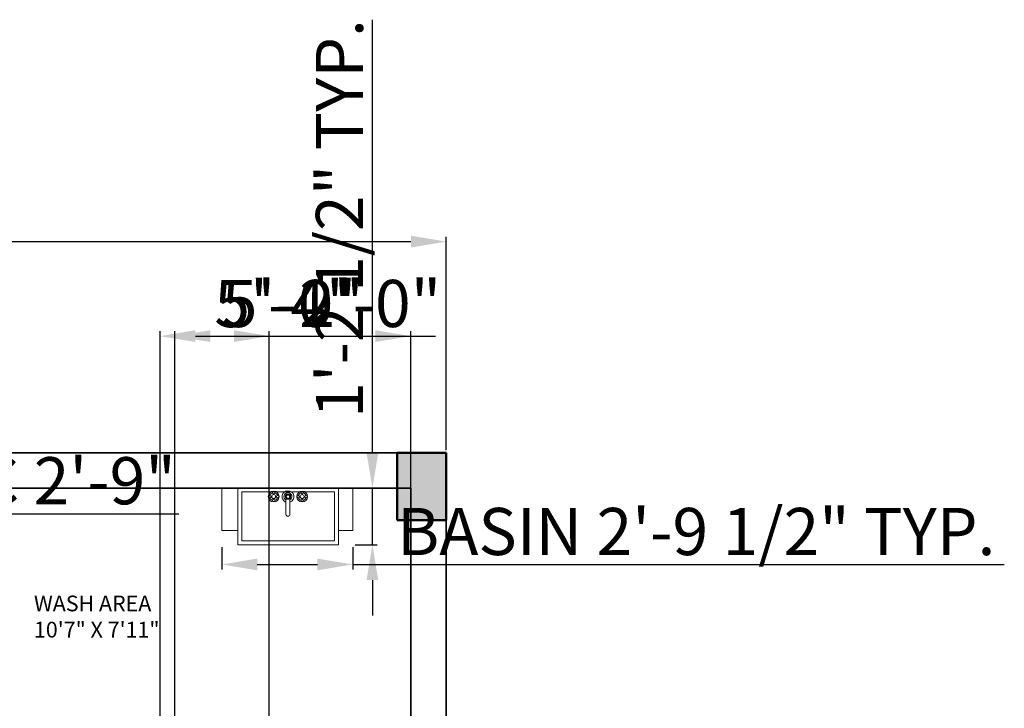
# Model space of a CAD drawing. Units: inches. Extents: x 1132 to 1713, y 3115 to 3781.
# Tile 4 of 4: x 1455 to 1705, y 3606 to 3781. Entities that reach past the tile are written whole.
import ezdxf

# ---------------------------------------------------------------- set-up
doc = ezdxf.new("R2010")
doc.units = ezdxf.units.IN
for name, color, linetype, lineweight in [('A-ANNO-DIMS', 2, 'Continuous', 18), ('A-AREA-IDEN', 7, 'Continuous', 18), ('A-COLS', 1, 'Continuous', 50), ('A-COLS-PATT', 252, 'Continuous', 13), ('A-FLOR-FIXT', 9, 'Continuous', 18), ('A-WALL', 7, 'Continuous', 35)]:
    doc.layers.add(name, color=color, linetype=linetype, lineweight=lineweight)
doc.styles.get("Standard").update_dxf_attribs({"font": 'arial.ttf'})
doc.dimstyles.new('ISO-25', dxfattribs={"dimtxt": 12, "dimasz": 9, "dimexe": 1.25, "dimexo": 0.625, "dimtad": 1, "dimdec": 0, "dimrnd": 2, "dimlunit": 3, "dimtxsty": 'Standard', "dimcen": 2.5, "dimadec": 0, "dimazin": 0, "dimtfac": 1, "dimtdec": 0, "dimtmove": 0, "dimatfit": 3, "dimfxl": 1, "dimarcsym": 0})

# ---------------------------------------------------------------- blocks, each defined once
blk = doc.blocks.new('*D19')
at = {"layer": 'A-ANNO-DIMS', "color": 0, "lineweight": -2, "transparency": 16777216}
for p, q in [((1268.16, 3667), (1268.16, 3725.86)), ((1563.22, 3671.51), (1563.22, 3725.86)), ((1277.16, 3724.61), (1554.22, 3724.61))]:
    blk.add_line(p, q, dxfattribs=at)
at = {"layer": 'A-ANNO-DIMS', "color": 0, "transparency": 16777216}
for points in [[(1277.16, 3726.11), (1277.16, 3723.11), (1268.16, 3724.61)], [(1554.22, 3726.11), (1554.22, 3723.11), (1563.22, 3724.61)]]:
    blk.add_solid(points, dxfattribs=at)
at = {"layer": 'Defpoints', "color": 0, "transparency": 16777216}
for p in [(1563.22, 3724.61), (1563.22, 3670.89), (1268.16, 3666.38)]:
    blk.add_point(p, dxfattribs=at)
at = {"layer": 'A-ANNO-DIMS', "color": 0, "transparency": 16777216, "insert": (1415.69, 3731.36), "char_height": 12, "attachment_point": 5}
blk.add_mtext('24\'-8"', dxfattribs=at)
blk = doc.blocks.new('Faucet - Bathroom top')
for p, q in [((-4.107, 0.125), (-4.375, 0.125)), ((-3.75, 0.4788), (-3.75, 0.75)), ((-3.5, 0.482), (-3.5, 0.75)), ((-3.1461, 0.125), (-2.875, 0.125)), ((3.143, 0.125), (2.875, 0.125)), ((3.5, 0.4788), (3.5, 0.75)), ((3.75, 0.482), (3.75, 0.75)), ((4.1039, 0.125), (4.375, 0.125)), ((-4.1039, -0.125), (-4.375, -0.125)), ((-3.75, -0.4821), (-3.75, -0.75)), ((-3.5, -0.4789), (-3.5, -0.75)), ((-3.143, -0.125), (-2.875, -0.125)), ((-0.5, -0.8639), (-0.5, -4.5)), ((0.5, -4.5), (0.5, -0.8631)), ((3.1461, -0.125), (2.875, -0.125)), ((3.5, -0.4821), (3.5, -0.75)), ((3.75, -0.4789), (3.75, -0.75)), ((4.107, -0.125), (4.375, -0.125))]:
    blk.add_line(p, q)
for centre, radius in [((-3.625, 0), 1.375), ((-4.625, 0), 0.2795), ((-3.625, 0), 0.5), ((-3.625, 1), 0.2795), ((-2.625, 0), 0.2795), ((0, 0), 0.5), ((3.625, 0), 1.375), ((2.625, 0), 0.2795), ((3.625, 0), 0.5), ((3.625, 1), 0.2795), ((4.625, 0), 0.2795), ((-3.625, -1), 0.2795), ((3.625, -1), 0.2795)]:
    blk.add_circle(centre, radius)
for centre, radius, start, end in [((-3.625, 0), 1, 105.2407, 164.2093), ((-3.625, 0), 1, 16.44125, 74.07887), ((0, 0), 1.5, 289.6514, 250.3603), ((0, 0), 1, 300.3431, 239.7554), ((3.625, 0), 1, 106.12, 164.0884), ((3.625, 0), 1, 16.23422, 73.90469), ((-3.625, 0), 1, 196.2342, 253.9047), ((-3.625, 0), 1, 286.12, 344.0884), ((3.625, 0), 1, 196.4413, 254.0789), ((3.625, 0), 1, 285.2407, 344.2093), ((0, -4.5), 0.5, 180, 0)]:
    blk.add_arc(centre, radius, start, end)
blk = doc.blocks.new('LAVATORY-WALL-MOUNT')
for p, q in [((-16.8, 2.17), (-16.8, -8.61)), ((16.5, -8.61), (16.5, 2.17)), ((-16.8, -8.61), (-12.71, -8.61)), ((12.88, -8.61), (16.5, -8.61))]:
    blk.add_line(p, q)
for points in [[(-12.71, 2.17), (12.88, 2.17), (12.88, -12.27), (-12.71, -12.27)], [(-11.71, 1.17), (11.88, 1.17), (11.88, -11.27), (-11.71, -11.27)]]:
    blk.add_lwpolyline(points, close=True)
for radius in [0.667, 0.447]:
    blk.add_circle((0, 0), radius)
blk.add_blockref('Faucet - Bathroom top', (0, 0))
blk = doc.blocks.new('*D28')
at = {"layer": 'A-ANNO-DIMS', "color": 0, "lineweight": -2, "transparency": 16777216}
for p, q in [((1506.13, 3646.81), (1506.13, 3641.19)), ((1539.42, 3646.81), (1539.42, 3641.19)), ((1515.13, 3642.44), (1530.42, 3642.44)), ((1539.42, 3642.44), (1705.22, 3642.44))]:
    blk.add_line(p, q, dxfattribs=at)
at = {"layer": 'A-ANNO-DIMS', "color": 0, "transparency": 16777216}
for points in [[(1515.13, 3643.94), (1515.13, 3640.94), (1506.13, 3642.44)], [(1530.42, 3643.94), (1530.42, 3640.94), (1539.42, 3642.44)]]:
    blk.add_solid(points, dxfattribs=at)
at = {"layer": 'Defpoints', "color": 0, "transparency": 16777216}
for p in [(1506.13, 3647.44), (1539.42, 3647.44), (1539.42, 3642.44)]:
    blk.add_point(p, dxfattribs=at)
at = {"layer": 'A-ANNO-DIMS', "color": 0, "transparency": 16777216, "insert": (1626.82, 3649.27), "char_height": 12, "attachment_point": 5}
blk.add_mtext('BASIN 2\'-9 1/2" TYP.', dxfattribs=at)
blk = doc.blocks.new('*D29')
at = {"layer": 'A-ANNO-DIMS', "color": 0, "lineweight": -2, "transparency": 16777216}
for p, q in [((1544.42, 3670.88), (1544.42, 3781.1)), ((1540.05, 3661.88), (1545.67, 3661.88)), ((1544.42, 3647.44), (1544.42, 3661.88)), ((1540.05, 3647.44), (1545.67, 3647.44)), ((1544.42, 3638.44), (1544.42, 3629.44))]:
    blk.add_line(p, q, dxfattribs=at)
at = {"layer": 'A-ANNO-DIMS', "color": 0, "transparency": 16777216}
for points in [[(1542.92, 3670.88), (1545.92, 3670.88), (1544.42, 3661.88)], [(1542.92, 3638.44), (1545.92, 3638.44), (1544.42, 3647.44)]]:
    blk.add_solid(points, dxfattribs=at)
at = {"layer": 'Defpoints', "color": 0, "transparency": 16777216}
for p in [(1539.42, 3661.88), (1544.42, 3661.88), (1539.42, 3647.44)]:
    blk.add_point(p, dxfattribs=at)
at = {"layer": 'A-ANNO-DIMS', "color": 0, "transparency": 16777216, "insert": (1537.59, 3730.49), "char_height": 12, "attachment_point": 5, "rotation": 90}
blk.add_mtext('1\'-2 1/2" TYP.', dxfattribs=at)
blk = doc.blocks.new('*D36')
at = {"layer": 'A-ANNO-DIMS', "color": 0, "lineweight": -2, "transparency": 16777216}
for p, q in [((1386.9, 3651.03), (1386.9, 3656.61)), ((1419.95, 3651.03), (1419.95, 3656.61)), ((1395.9, 3655.36), (1410.95, 3655.36)), ((1419.95, 3655.36), (1495.17, 3655.36))]:
    blk.add_line(p, q, dxfattribs=at)
at = {"layer": 'A-ANNO-DIMS', "color": 0, "transparency": 16777216}
for points in [[(1395.9, 3656.86), (1395.9, 3653.86), (1386.9, 3655.36)], [(1410.95, 3656.86), (1410.95, 3653.86), (1419.95, 3655.36)]]:
    blk.add_solid(points, dxfattribs=at)
at = {"layer": 'Defpoints', "color": 0, "transparency": 16777216}
for p in [(1419.95, 3655.36), (1386.9, 3650.4), (1419.95, 3650.4)]:
    blk.add_point(p, dxfattribs=at)
at = {"layer": 'A-ANNO-DIMS', "color": 0, "transparency": 16777216, "insert": (1462.06, 3662.19), "char_height": 12, "attachment_point": 5}
blk.add_mtext('WC 2\'-9"', dxfattribs=at)
blk = doc.blocks.new('*D50')
at = {"layer": 'A-ANNO-DIMS', "color": 0, "lineweight": -2, "transparency": 16777216}
for p, q in [((1490.38, 3260.74), (1490.38, 3701.81)), ((1554.16, 3217.5), (1554.16, 3701.81)), ((1499.38, 3700.56), (1545.16, 3700.56))]:
    blk.add_line(p, q, dxfattribs=at)
at = {"layer": 'A-ANNO-DIMS', "color": 0, "transparency": 16777216}
for points in [[(1499.38, 3702.06), (1499.38, 3699.06), (1490.38, 3700.56)], [(1545.16, 3702.06), (1545.16, 3699.06), (1554.16, 3700.56)]]:
    blk.add_solid(points, dxfattribs=at)
at = {"layer": 'Defpoints', "color": 0, "transparency": 16777216}
for p in [(1554.16, 3700.56), (1490.38, 3260.12), (1554.16, 3216.88)]:
    blk.add_point(p, dxfattribs=at)
at = {"layer": 'A-ANNO-DIMS', "color": 0, "transparency": 16777216, "insert": (1522.27, 3707.29), "char_height": 12, "attachment_point": 5}
blk.add_mtext('5\'-4"', dxfattribs=at)
blk = doc.blocks.new('*D55')
at = {"layer": 'A-ANNO-DIMS', "color": 0, "lineweight": -2, "transparency": 16777216}
for p, q in [((1494.16, 3463.5), (1494.16, 3701.81)), ((1554.16, 3463.5), (1554.16, 3701.81)), ((1503.16, 3700.56), (1545.16, 3700.56))]:
    blk.add_line(p, q, dxfattribs=at)
at = {"layer": 'A-ANNO-DIMS', "color": 0, "transparency": 16777216}
for points in [[(1503.16, 3702.06), (1503.16, 3699.06), (1494.16, 3700.56)], [(1545.16, 3702.06), (1545.16, 3699.06), (1554.16, 3700.56)]]:
    blk.add_solid(points, dxfattribs=at)
at = {"layer": 'Defpoints', "color": 0, "transparency": 16777216}
for p in [(1554.16, 3700.56), (1494.16, 3462.88), (1554.16, 3462.88)]:
    blk.add_point(p, dxfattribs=at)
at = {"layer": 'A-ANNO-DIMS', "color": 0, "transparency": 16777216, "insert": (1524.16, 3707.31), "char_height": 12, "attachment_point": 5}
blk.add_mtext('5\'-0"', dxfattribs=at)
blk = doc.blocks.new('*D58')
at = {"layer": 'A-ANNO-DIMS', "color": 0, "lineweight": -2, "transparency": 16777216}
for p, q in [((1494.16, 3487.5), (1494.16, 3701.81)), ((1518.16, 3487.5), (1518.16, 3701.81)), ((1503.16, 3700.56), (1509.16, 3700.56)), ((1518.16, 3700.56), (1560.51, 3700.56))]:
    blk.add_line(p, q, dxfattribs=at)
at = {"layer": 'A-ANNO-DIMS', "color": 0, "transparency": 16777216}
for points in [[(1503.16, 3702.06), (1503.16, 3699.06), (1494.16, 3700.56)], [(1509.16, 3702.06), (1509.16, 3699.06), (1518.16, 3700.56)]]:
    blk.add_solid(points, dxfattribs=at)
at = {"layer": 'Defpoints', "color": 0, "transparency": 16777216}
for p in [(1518.16, 3700.56), (1494.16, 3486.88), (1518.16, 3486.88)]:
    blk.add_point(p, dxfattribs=at)
at = {"layer": 'A-ANNO-DIMS', "color": 0, "transparency": 16777216, "insert": (1543.84, 3707.31), "char_height": 12, "attachment_point": 5}
blk.add_mtext('2\'-0"', dxfattribs=at)

msp = doc.modelspace()

# ---------------------------------------------------------------- hatches: boundary and pattern name
at = {"layer": 'A-COLS-PATT'}
h = msp.add_hatch(color=256, dxfattribs=at)
h.dxf.hatch_style = 1
h.paths.add_polyline_path([(1563.16, 3670.88), (1550.72, 3670.88), (1550.72, 3661.88), (1554.16, 3661.88), (1554.16, 3653.71), (1563.16, 3653.71)])
h = msp.add_hatch(color=256, dxfattribs=at)
h.dxf.hatch_style = 1
h.paths.add_polyline_path([(1550.72, 3653.71), (1554.16, 3653.71), (1554.16, 3661.88), (1550.72, 3661.88)])

# ---------------------------------------------------------------- linework, layer by layer
at = {"layer": 'A-COLS'}
for p, q in [((1550.72, 3670.89), (1563.22, 3670.89)), ((1550.72, 3653.71), (1550.72, 3670.89)), ((1563.22, 3670.89), (1563.22, 3653.71)), ((1563.22, 3653.71), (1550.72, 3653.71))]:
    msp.add_line(p, q, dxfattribs=at)
at = {"layer": 'A-WALL'}
for p, q in [((1430.16, 3661.88), (1554.16, 3661.88)), ((1554.16, 3661.88), (1554.16, 3566.88))]:
    msp.add_line(p, q, dxfattribs=at)
msp.add_lwpolyline([(1268.16, 3670.88), (1563.16, 3670.88), (1563.16, 3145.88), (1268.16, 3145.88)], close=True, dxfattribs=at)

# ---------------------------------------------------------------- block references
at = {"layer": 'A-FLOR-FIXT'}
msp.add_blockref('LAVATORY-WALL-MOUNT', (1522.92, 3659.71), dxfattribs=at)

# ---------------------------------------------------------------- texts
at = {"layer": 'A-AREA-IDEN', "insert": (1458.29, 3634.51), "char_height": 4, "attachment_point": 1}
msp.add_mtext_dynamic_manual_height_columns('{\\fArial|b1|i0|c0|p34;WASH AREA\\P10\'7" X 7\'11"}', width=83.7568, gutter_width=12.5, heights=[54.87], dxfattribs=at)

# ---------------------------------------------------------------- dimensions: what is measured, and where the dimension line sits
at = {"layer": 'A-ANNO-DIMS'}
dim = msp.add_linear_dim(base=(1544.42, 3661.88), p1=(1539.42, 3647.44), p2=(1539.42, 3661.88), angle=90, text='<> TYP.', dimstyle='ISO-25', override={"dimdec": 1, "dimlfac": 1, "dimrnd": 0, "dimzin": 1, "dimdsep": 46, "dimlunit": 4, "dimfrac": 2}, dxfattribs=at)
dim.commit()
dim.dimension.update_dxf_attribs({"geometry": '*D29', "text_midpoint": (1537.59, 3730.49)})
for base, p1, p2, override, picture, middle in [((1563.22, 3724.61), (1268.16, 3666.38), (1563.22, 3670.89), {"dimclrd": 0, "dimclre": 0, "dimclrt": 0}, '*D19', (1415.69, 3731.36)), ((1554.16, 3700.56), (1490.38, 3260.12), (1554.16, 3216.88), {"dimdec": 1, "dimlfac": 1, "dimrnd": 0, "dimzin": 1, "dimdsep": 46, "dimlunit": 4, "dimfrac": 2}, '*D50', (1522.27, 3707.29)), ((1554.16, 3700.56), (1494.16, 3462.88), (1554.16, 3462.88), {"dimdec": 1, "dimlfac": 1, "dimrnd": 0, "dimzin": 1, "dimdsep": 46, "dimlunit": 4, "dimfrac": 2}, '*D55', (1524.16, 3707.31)), ((1518.16, 3700.56), (1494.16, 3486.88), (1518.16, 3486.88), {"dimdec": 1, "dimlfac": 1, "dimrnd": 0, "dimzin": 1, "dimdsep": 46, "dimlunit": 4, "dimfrac": 2}, '*D58', (1543.84, 3707.31))]:
    dim = msp.add_linear_dim(base=base, p1=p1, p2=p2, dimstyle='ISO-25', override=override, dxfattribs=at)
    dim.commit()
    dim.dimension.update_dxf_attribs({"geometry": picture, "text_midpoint": middle})
for base, p1, p2, text, picture, middle in [((1539.42, 3642.44), (1506.13, 3647.44), (1539.42, 3647.44), 'BASIN <> TYP.', '*D28', (1626.82, 3649.27)), ((1419.9459, 3655.3614), (1386.8997, 3650.4044), (1419.9459, 3650.4044), 'WC <>', '*D36', (1462.0593, 3662.191))]:
    dim = msp.add_linear_dim(base=base, p1=p1, p2=p2, text=text, dimstyle='ISO-25', override={"dimdec": 1, "dimlfac": 1, "dimrnd": 0, "dimzin": 1, "dimdsep": 46, "dimlunit": 4, "dimfrac": 2}, dxfattribs=at)
    dim.commit()
    dim.dimension.update_dxf_attribs({"geometry": picture, "text_midpoint": middle})

doc.saveas('drawing.dxf')
